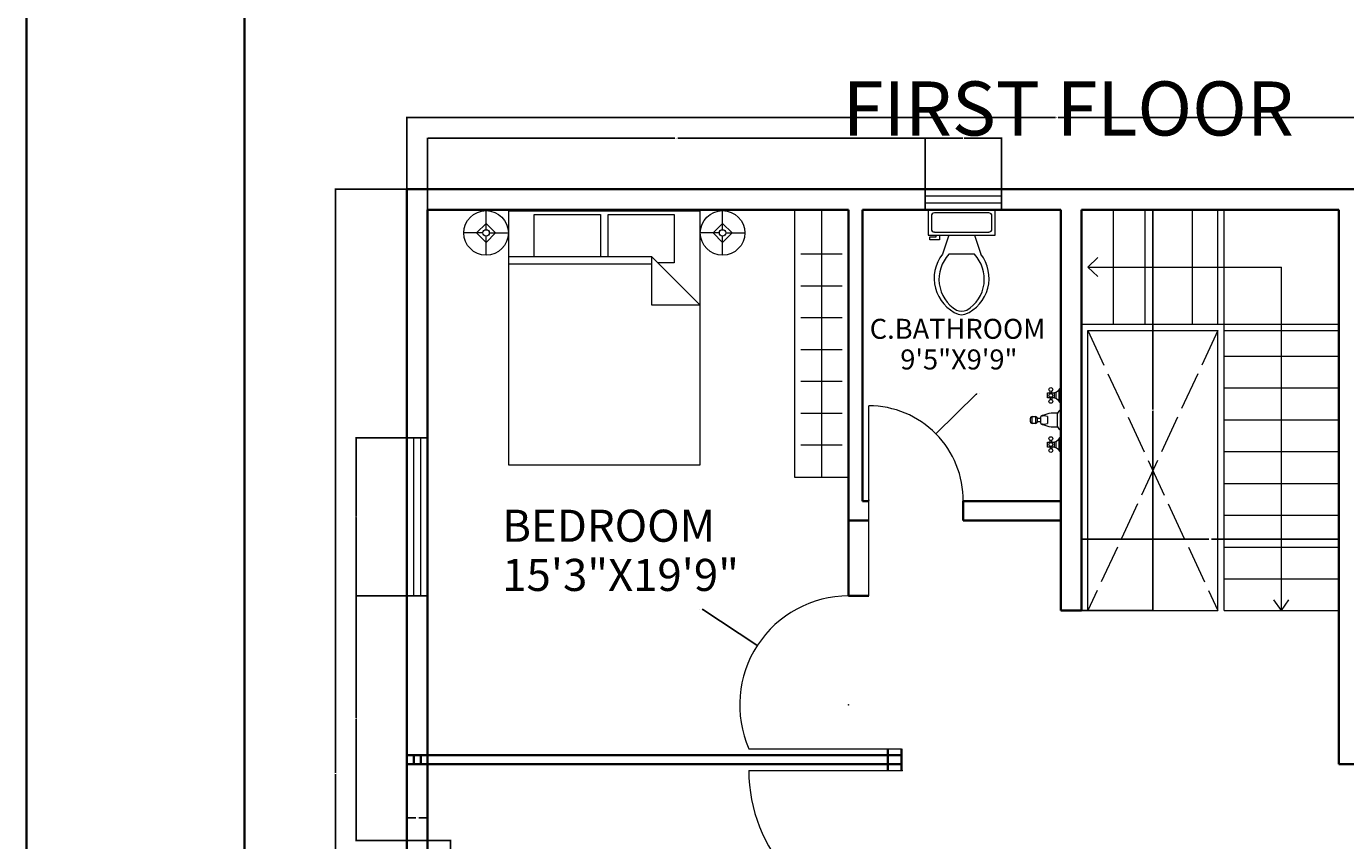
# Model space of a CAD drawing. Units: inches. Extents: x 2286 to 3750, y 1240 to 2345.
# Tile 2 of 7: x 2286 to 2701, y 1537 to 1793. Entities that reach past the tile are written whole.
import ezdxf

# ---------------------------------------------------------------- set-up
doc = ezdxf.new("R2010")
doc.units = ezdxf.units.IN
doc.linetypes.add('ACAD_ISO02W100', pattern=[15, 12, -3])
for name, color, linetype, lineweight in [('A-ANNO-DIMS', 2, 'Continuous', 18), ('A-ANNO-TEXT', 7, 'Continuous', 35), ('A-AREA-IDEN', 7, 'Continuous', 18), ('A-DOOR', 4, 'Continuous', 18), ('A-FLOR-CASE', 8, 'Continuous', 18), ('A-FLOR-FIXT', 9, 'Continuous', 18), ('A-FLOR-STRS', 7, 'Continuous', 18), ('A-FLOR-STRS-HIDN', 8, 'ACAD_ISO02W100', 13), ('A-FURN', 8, 'Continuous', 18), ('A-GLAZ', 51, 'Continuous', 18), ('A-WALL', 7, 'Continuous', 35)]:
    doc.layers.add(name, color=color, linetype=linetype, lineweight=lineweight)
doc.styles.get("Standard").update_dxf_attribs({"font": 'arial.ttf'})
doc.dimstyles.get("Standard").update_dxf_attribs({"dimtxt": 0.18, "dimasz": 0.18, "dimexe": 0.18, "dimexo": 0.0625, "dimgap": 0.09, "dimtad": 0, "dimtih": 1, "dimtoh": 1, "dimdec": 4, "dimzin": 0, "dimdsep": 46, "dimtxsty": 'Standard', "dimcen": 0.09, "dimadec": 0, "dimazin": 0, "dimtfac": 1, "dimtdec": 4, "dimtofl": 0, "dimtmove": 0, "dimatfit": 3, "dimfxl": 1, "dimtolj": 1, "dimtzin": 0, "dimarcsym": 0})

# ---------------------------------------------------------------- blocks, each defined once
blk = doc.blocks.new('Toilet - top')
for p, q in [((9.5, -6), (9.5, -2)), ((-8, -8.5), (-8, -8)), ((-7, -8), (-7, -9.5)), ((-4, -8), (-6, -14)), ((4, -8), (6, -14)), ((-10, -8.5), (-8, -8.5)), ((-10, -9.5), (-10, -8.5)), ((-7, -9.5), (-10, -9.5)), ((4, -14), (-4, -14))]:
    blk.add_line(p, q)
blk.add_lwpolyline([(10.5, -8), (10.5, 0), (-10.5, 0), (-10.5, -8)], close=True)
for points in [[(-9.5, -2), (-9.5, -6)], [(8.5, -1), (-8.5, -1)], [(-8.5, -7), (8.5, -7)]]:
    blk.add_lwpolyline(points)
for centre, radius, start, end in [((-8.62, -1.88), 0.884, 81.8699, 188.1301), ((8.62, -1.88), 0.884, 351.8699, 98.1301), ((-8.62, -6.12), 0.884, 171.8699, 278.1301), ((8.62, -6.12), 0.884, 261.8699, 8.1301), ((3.52, -21.58), 12.17, 141.4691, 247.9714), ((4.2, -21.82), 11.33, 136.3677, 238.9468), ((-3.52, -21.58), 12.17, 292.0284, 38.5307), ((-4.2, -21.82), 11.33, 301.053, 43.6321), ((0, -27.88), 4, 245.7318, 294.2682), ((0, -29), 4, 254.8605, 285.1395)]:
    blk.add_arc(centre, radius, start, end)
blk = doc.blocks.new('Bed - Queen')
for p, q in [((0, -80.00003), (0, 0)), ((0, 0), (59.99999, 0)), ((59.99999, 0), (59.99999, -80.00003)), ((7.99999, -1.2), (28.79998, -1.2)), ((7.99999, -14.4), (7.99999, -1.2)), ((28.79998, -1.2), (28.79998, -14.4)), ((31.19999, -1.2), (51.99999, -1.2)), ((31.19999, -14.4), (31.19999, -1.2)), ((51.99999, -1.2), (51.99999, -16.4)), ((0, -14.4), (44.8, -14.4)), ((59.99999, -29.6), (44.8, -14.4)), ((44.8, -14.4), (44.8, -29.6)), ((51.99999, -16.4), (46.79936, -16.4)), ((44.8, -16.8), (0, -16.8)), ((44.8, -29.6), (59.99999, -29.6)), ((59.99999, -80.00003), (0, -80.00003))]:
    blk.add_line(p, q)
blk = doc.blocks.new('Lamp - Table')
for p, q in [((0, 7), (0, 1)), ((-1, 0), (-7, 0)), ((0, 3), (-3, 0)), ((-3, 0), (0, -3)), ((3, 0), (0, 3)), ((0, -3), (3, 0)), ((1, 0), (7, 0)), ((0, -1), (0, -7))]:
    blk.add_line(p, q)
for radius in [7, 1]:
    blk.add_circle((0, 0), radius)
blk = doc.blocks.new('Faucet - Bathroom front')
for p, q in [((-0.5, 4.25), (0.5, 4.25)), ((0.5, 3.75), (-0.5, 3.75)), ((-0.5, 3), (0.5, 3)), ((0.5, 2), (-0.5, 2)), ((-0.25, 3), (-0.25, 3.5)), ((0.25, 3.5), (0.25, 3)), ((-5, 0), (-2.25, 0)), ((-4.5087, 0.25), (-2.7408, 0.25)), ((-4, 1.625), (-4.25, 1.625)), ((-4, 1.375), (-4.25, 1.375)), ((-3.1442, 0.75), (-4.0979, 0.75)), ((-3.25, 1.625), (-3, 1.625)), ((-3.25, 1.375), (-3, 1.375)), ((-1.5, 0), (1.5, 0)), ((-1, 0.5), (1, 0.5)), ((2.25, 0), (5, 0)), ((2.7413, 0.25), (4.5092, 0.25)), ((3.25, 1.625), (3, 1.625)), ((3.25, 1.375), (3, 1.375)), ((4.1058, 0.75), (3.1521, 0.75)), ((4, 1.625), (4.25, 1.625)), ((4, 1.375), (4.25, 1.375))]:
    blk.add_line(p, q)
for points in [[(-0.5, 3.75), (-0.5, 4.25)], [(-0.25, 4.5), (0.25, 4.5)], [(0.5, 4.25), (0.5, 3.75)], [(0.25, 3.5), (-0.25, 3.5)]]:
    blk.add_lwpolyline(points)
for points in [[(-4, 1), (-4, 2), (-3.25, 2), (-3.25, 1)], [(3.25, 1), (3.25, 2), (4, 2), (4, 1)]]:
    blk.add_lwpolyline(points, close=True)
for centre in [(-4.5, 1.5), (-3.625, 1.5), (-2.75, 1.5), (2.75, 1.5), (3.625, 1.5), (4.5, 1.5)]:
    blk.add_circle(centre, 0.2795)
for centre, radius, start, end in [((-0.2575, 4.2575), 0.2426, 88.22243, 181.7776), ((0.2575, 4.2575), 0.2426, 358.2224, 91.77757), ((3, 1), 4.0311, 150.2551, 187.125), ((0.6413, 2.5), 1.246, 156.3417, 203.6583), ((-0.2575, 3.7425), 0.2426, 178.2224, 271.7776), ((0.2575, 3.7425), 0.2426, 268.2224, 1.777565), ((-3, 1), 4.0311, 352.875, 29.74488), ((-0.6413, 2.5), 1.246, 336.3417, 23.65835), ((-5.375, 1.375), 1.4252, 285.2551, 344.7449), ((-1.875, 1.375), 1.4252, 195.2551, 254.7449), ((-0.7962, -0.2038), 0.7327, 106.1502, 163.8498), ((0.7962, -0.2038), 0.7327, 16.1502, 73.84979), ((1.875, 1.375), 1.4252, 285.2551, 344.7449), ((5.375, 1.375), 1.4252, 195.2551, 254.7449)]:
    blk.add_arc(centre, radius, start, end)
blk = doc.blocks.new('CLOSET-RAIL-84')
for p, q in [((6.5, 0), (6.5, 84)), ((0, 74), (13, 74)), ((0, 64), (13, 64)), ((0, 54), (13, 54)), ((0, 44), (13, 44)), ((0, 34), (13, 34)), ((0, 24), (13, 24)), ((0, 14), (13, 14))]:
    blk.add_line(p, q)
blk = doc.blocks.new('*D36')
at = {"layer": 'A-ANNO-DIMS', "color": 0, "lineweight": -2, "transparency": 16777216}
for p, q in [((2412.36, 1536.75), (2419.68, 1536.75)), ((2419.5, 1536.57), (2419.5, 1512.93)), ((2419.5, 1488.93), (2419.5, 1512.56)), ((2412.36, 1488.75), (2419.68, 1488.75))]:
    blk.add_line(p, q, dxfattribs=at)
at = {"layer": 'A-ANNO-DIMS', "color": 0, "transparency": 16777216}
for points in [[(2419.47, 1536.57), (2419.53, 1536.57), (2419.5, 1536.75)], [(2419.47, 1488.93), (2419.53, 1488.93), (2419.5, 1488.75)]]:
    blk.add_solid(points, dxfattribs=at)
at = {"layer": 'Defpoints', "color": 0, "transparency": 16777216}
for p in [(2412.3, 1536.75), (2419.5, 1536.75), (2412.3, 1488.75)]:
    blk.add_point(p, dxfattribs=at)
at = {"layer": 'A-ANNO-DIMS', "color": 0, "transparency": 16777216, "insert": (2419.5, 1512.75), "char_height": 0.18, "attachment_point": 5}
blk.add_mtext('\\A1;WINDOW 48 TYP.', dxfattribs=at)
blk = doc.blocks.new('*D37')
at = {"layer": 'A-ANNO-DIMS', "color": 0, "lineweight": -2, "transparency": 16777216}
for p, q in [((2405.79, 1536.81), (2405.79, 1544.13)), ((2405.97, 1543.95), (2408.59, 1543.95)), ((2412.12, 1543.95), (2409.5, 1543.95)), ((2412.3, 1536.81), (2412.3, 1544.13))]:
    blk.add_line(p, q, dxfattribs=at)
at = {"layer": 'A-ANNO-DIMS', "color": 0, "transparency": 16777216}
for points in [[(2405.97, 1543.98), (2405.97, 1543.92), (2405.79, 1543.95)], [(2412.12, 1543.98), (2412.12, 1543.92), (2412.3, 1543.95)]]:
    blk.add_solid(points, dxfattribs=at)
at = {"layer": 'Defpoints', "color": 0, "transparency": 16777216}
for p in [(2405.79, 1543.95), (2405.79, 1536.75), (2412.3, 1536.75)]:
    blk.add_point(p, dxfattribs=at)
at = {"layer": 'A-ANNO-DIMS', "color": 0, "transparency": 16777216, "insert": (2409.04, 1543.95), "char_height": 0.18, "attachment_point": 5}
blk.add_mtext('\\A1;7 TYP.', dxfattribs=at)
blk = doc.blocks.new('*D75')
at = {"layer": 'A-ANNO-DIMS', "color": 0, "lineweight": -2, "transparency": 16777216}
for p, q in [((2405.73, 1741.53), (2383.16, 1741.53)), ((2383.34, 1741.35), (2383.34, 1558.04)), ((2383.34, 1374.36), (2383.34, 1557.67)), ((2405.73, 1374.18), (2383.16, 1374.18))]:
    blk.add_line(p, q, dxfattribs=at)
at = {"layer": 'A-ANNO-DIMS', "color": 0, "transparency": 16777216}
for points in [[(2383.31, 1741.35), (2383.37, 1741.35), (2383.34, 1741.53)], [(2383.31, 1374.36), (2383.37, 1374.36), (2383.34, 1374.18)]]:
    blk.add_solid(points, dxfattribs=at)
at = {"layer": 'Defpoints', "color": 0, "transparency": 16777216}
for p in [(2383.34, 1741.53), (2405.79, 1741.53), (2405.79, 1374.18)]:
    blk.add_point(p, dxfattribs=at)
at = {"layer": 'A-ANNO-DIMS', "color": 0, "transparency": 16777216, "insert": (2383.34, 1557.85), "char_height": 0.18, "attachment_point": 5}
blk.add_mtext('\\A1;367.35', dxfattribs=at)
blk = doc.blocks.new('*D76')
at = {"layer": 'A-ANNO-DIMS', "color": 0, "lineweight": -2, "transparency": 16777216}
for p, q in [((2405.79, 1741.59), (2405.79, 1764.22)), ((2405.97, 1764.04), (2609.67, 1764.04)), ((2814.17, 1764.04), (2610.47, 1764.04)), ((2814.35, 1741.59), (2814.35, 1764.22))]:
    blk.add_line(p, q, dxfattribs=at)
at = {"layer": 'A-ANNO-DIMS', "color": 0, "transparency": 16777216}
for points in [[(2405.97, 1764.07), (2405.97, 1764.01), (2405.79, 1764.04)], [(2814.17, 1764.07), (2814.17, 1764.01), (2814.35, 1764.04)]]:
    blk.add_solid(points, dxfattribs=at)
at = {"layer": 'Defpoints', "color": 0, "transparency": 16777216}
for p in [(2814.35, 1764.04), (2405.79, 1741.53), (2814.35, 1741.53)]:
    blk.add_point(p, dxfattribs=at)
at = {"layer": 'A-ANNO-DIMS', "color": 0, "transparency": 16777216, "insert": (2610.07, 1764.04), "char_height": 0.18, "attachment_point": 5}
blk.add_mtext('\\A1;408.6', dxfattribs=at)
blk = doc.blocks.new('*D78')
at = {"layer": 'A-ANNO-DIMS', "color": 0, "lineweight": -2, "transparency": 16777216}
for p, q in [((2617.83, 1609.08), (2617.83, 1631.65)), ((2618.01, 1631.47), (2657.85, 1631.47)), ((2698.47, 1631.47), (2658.64, 1631.47)), ((2698.65, 1609.08), (2698.65, 1631.65))]:
    blk.add_line(p, q, dxfattribs=at)
at = {"layer": 'A-ANNO-DIMS', "color": 0, "transparency": 16777216}
for points in [[(2618.01, 1631.5), (2618.01, 1631.44), (2617.83, 1631.47)], [(2698.47, 1631.5), (2698.47, 1631.44), (2698.65, 1631.47)]]:
    blk.add_solid(points, dxfattribs=at)
at = {"layer": 'Defpoints', "color": 0, "transparency": 16777216}
for p in [(2698.65, 1631.47), (2617.83, 1609.02), (2698.65, 1609.02)]:
    blk.add_point(p, dxfattribs=at)
at = {"layer": 'A-ANNO-DIMS', "color": 0, "transparency": 16777216, "insert": (2658.24, 1631.47), "char_height": 0.18, "attachment_point": 5}
blk.add_mtext('\\A1;80.82', dxfattribs=at)
blk = doc.blocks.new('*D79')
at = {"layer": 'A-ANNO-DIMS', "color": 0, "lineweight": -2, "transparency": 16777216}
for p, q in [((2617.89, 1735.02), (2640.46, 1735.02)), ((2640.28, 1734.84), (2640.28, 1672.2)), ((2640.28, 1609.2), (2640.28, 1671.84)), ((2617.89, 1609.02), (2640.46, 1609.02))]:
    blk.add_line(p, q, dxfattribs=at)
at = {"layer": 'A-ANNO-DIMS', "color": 0, "transparency": 16777216}
for points in [[(2640.25, 1734.84), (2640.31, 1734.84), (2640.28, 1735.02)], [(2640.25, 1609.2), (2640.31, 1609.2), (2640.28, 1609.02)]]:
    blk.add_solid(points, dxfattribs=at)
at = {"layer": 'Defpoints', "color": 0, "transparency": 16777216}
for p in [(2617.83, 1735.02), (2617.83, 1609.02), (2640.28, 1609.02)]:
    blk.add_point(p, dxfattribs=at)
at = {"layer": 'A-ANNO-DIMS', "color": 0, "transparency": 16777216, "insert": (2640.28, 1672.02), "char_height": 0.18, "attachment_point": 5}
blk.add_mtext('\\A1;126', dxfattribs=at)
blk = doc.blocks.new('*D83')
at = {"layer": 'A-ANNO-DIMS', "color": 0, "lineweight": -2, "transparency": 16777216}
for p, q in [((2412.23, 1613.64), (2389.67, 1613.64)), ((2389.85, 1613.46), (2389.85, 1575.37)), ((2389.85, 1536.93), (2389.85, 1575.01)), ((2412.23, 1536.75), (2389.67, 1536.75))]:
    blk.add_line(p, q, dxfattribs=at)
at = {"layer": 'A-ANNO-DIMS', "color": 0, "transparency": 16777216}
for points in [[(2389.82, 1613.46), (2389.88, 1613.46), (2389.85, 1613.64)], [(2389.82, 1536.93), (2389.88, 1536.93), (2389.85, 1536.75)]]:
    blk.add_solid(points, dxfattribs=at)
at = {"layer": 'Defpoints', "color": 0, "transparency": 16777216}
for p in [(2389.85, 1613.64), (2412.3, 1613.64), (2412.3, 1536.75)]:
    blk.add_point(p, dxfattribs=at)
at = {"layer": 'A-ANNO-DIMS', "color": 0, "transparency": 16777216, "insert": (2389.85, 1575.19), "char_height": 0.18, "attachment_point": 5}
blk.add_mtext('\\A1;76.9', dxfattribs=at)
blk = doc.blocks.new('*D84')
at = {"layer": 'A-ANNO-DIMS', "color": 0, "lineweight": -2, "transparency": 16777216}
for p, q in [((2412.23, 1663.29), (2389.67, 1663.29)), ((2389.85, 1663.11), (2389.85, 1638.65)), ((2389.85, 1613.82), (2389.85, 1638.28)), ((2412.23, 1613.64), (2389.67, 1613.64))]:
    blk.add_line(p, q, dxfattribs=at)
at = {"layer": 'A-ANNO-DIMS', "color": 0, "transparency": 16777216}
for points in [[(2389.82, 1663.11), (2389.88, 1663.11), (2389.85, 1663.29)], [(2389.82, 1613.82), (2389.88, 1613.82), (2389.85, 1613.64)]]:
    blk.add_solid(points, dxfattribs=at)
at = {"layer": 'Defpoints', "color": 0, "transparency": 16777216}
for p in [(2389.85, 1663.29), (2412.3, 1663.29), (2412.3, 1613.64)]:
    blk.add_point(p, dxfattribs=at)
at = {"layer": 'A-ANNO-DIMS', "color": 0, "transparency": 16777216, "insert": (2389.85, 1638.47), "char_height": 0.18, "attachment_point": 5}
blk.add_mtext('\\A1;49.65', dxfattribs=at)
blk = doc.blocks.new('*D85')
at = {"layer": 'A-ANNO-DIMS', "color": 0, "lineweight": -2, "transparency": 16777216}
for p, q in [((2412.3, 1735.08), (2412.29, 1757.65)), ((2412.47, 1757.47), (2490.04, 1757.5)), ((2568.53, 1757.53), (2490.95, 1757.5)), ((2568.72, 1735.15), (2568.71, 1757.71))]:
    blk.add_line(p, q, dxfattribs=at)
at = {"layer": 'A-ANNO-DIMS', "color": 0, "transparency": 16777216}
for points in [[(2412.47, 1757.5), (2412.47, 1757.44), (2412.29, 1757.47)], [(2568.53, 1757.56), (2568.53, 1757.5), (2568.71, 1757.53)]]:
    blk.add_solid(points, dxfattribs=at)
at = {"layer": 'Defpoints', "color": 0, "transparency": 16777216}
for p in [(2568.71, 1757.53), (2412.3, 1735.02), (2568.72, 1735.08)]:
    blk.add_point(p, dxfattribs=at)
at = {"layer": 'A-ANNO-DIMS', "color": 0, "transparency": 16777216, "insert": (2490.5, 1757.5), "char_height": 0.18, "attachment_point": 5}
blk.add_mtext('\\A1;156.42', dxfattribs=at)
blk = doc.blocks.new('*D86')
at = {"layer": 'A-ANNO-DIMS', "color": 0, "lineweight": -2, "transparency": 16777216}
for p, q in [((2568.72, 1735.15), (2568.72, 1757.71)), ((2568.9, 1757.53), (2580.5, 1757.53)), ((2592.54, 1757.53), (2580.94, 1757.53)), ((2592.72, 1735.15), (2592.72, 1757.71))]:
    blk.add_line(p, q, dxfattribs=at)
at = {"layer": 'A-ANNO-DIMS', "color": 0, "transparency": 16777216}
for points in [[(2568.9, 1757.56), (2568.9, 1757.5), (2568.72, 1757.53)], [(2592.54, 1757.56), (2592.54, 1757.5), (2592.72, 1757.53)]]:
    blk.add_solid(points, dxfattribs=at)
at = {"layer": 'Defpoints', "color": 0, "transparency": 16777216}
for p in [(2592.72, 1757.53), (2568.72, 1735.08), (2592.72, 1735.08)]:
    blk.add_point(p, dxfattribs=at)
at = {"layer": 'A-ANNO-DIMS', "color": 0, "transparency": 16777216, "insert": (2580.72, 1757.53), "char_height": 0.18, "attachment_point": 5}
blk.add_mtext('\\A1;24', dxfattribs=at)
blk = doc.blocks.new('*D128')
at = {"layer": 'A-ANNO-DIMS', "color": 0, "lineweight": -2, "transparency": 16777216}
for p, q in [((2561.39, 1558.75), (2561.57, 1558.75)), ((2561.48, 1558.66), (2561.48, 1558.84)), ((2504.41, 1506.84), (2525.67, 1526.18)), ((2504.23, 1506.84), (2504.41, 1506.84))]:
    blk.add_line(p, q, dxfattribs=at)
at = {"layer": 'A-ANNO-DIMS', "color": 0, "transparency": 16777216}
blk.add_solid([(2525.65, 1526.2), (2525.69, 1526.16), (2525.81, 1526.3)], dxfattribs=at)
at = {"layer": 'Defpoints', "color": 0, "transparency": 16777216}
for p in [(2561.48, 1558.75), (2525.81, 1526.3)]:
    blk.add_point(p, dxfattribs=at)
at = {"layer": 'A-ANNO-DIMS', "color": 0, "transparency": 16777216, "insert": (2503.75, 1506.84), "char_height": 0.18, "attachment_point": 5}
blk.add_mtext('\\A1;R48.22', dxfattribs=at)
blk = doc.blocks.new('*D130')
at = {"layer": 'A-ANNO-DIMS', "color": 0, "lineweight": -2, "transparency": 16777216}
for p, q in [((2498.58, 1609.37), (2498.76, 1609.37)), ((2498.76, 1609.37), (2515.81, 1598.22)), ((2544.54, 1579.39), (2544.72, 1579.39)), ((2544.63, 1579.3), (2544.63, 1579.48))]:
    blk.add_line(p, q, dxfattribs=at)
at = {"layer": 'A-ANNO-DIMS', "color": 0, "transparency": 16777216}
blk.add_solid([(2515.82, 1598.25), (2515.79, 1598.2), (2515.96, 1598.13)], dxfattribs=at)
at = {"layer": 'Defpoints', "color": 0, "transparency": 16777216}
for p in [(2515.96, 1598.13), (2544.63, 1579.39)]:
    blk.add_point(p, dxfattribs=at)
at = {"layer": 'A-ANNO-DIMS', "color": 0, "transparency": 16777216, "insert": (2498.1, 1609.37), "char_height": 0.18, "attachment_point": 5}
blk.add_mtext('\\A1;R34.25', dxfattribs=at)
blk = doc.blocks.new('*D132')
at = {"layer": 'A-ANNO-DIMS', "color": 0, "lineweight": -2, "transparency": 16777216}
for p, q in [((2584.72, 1677.1), (2572.19, 1664.72)), ((2584.9, 1677.1), (2584.72, 1677.1)), ((2550.88, 1643.73), (2551.06, 1643.73)), ((2550.97, 1643.64), (2550.97, 1643.82))]:
    blk.add_line(p, q, dxfattribs=at)
at = {"layer": 'A-ANNO-DIMS', "color": 0, "transparency": 16777216}
blk.add_solid([(2572.17, 1664.74), (2572.21, 1664.69), (2572.06, 1664.59)], dxfattribs=at)
at = {"layer": 'Defpoints', "color": 0, "transparency": 16777216}
for p in [(2572.06, 1664.59), (2550.97, 1643.73)]:
    blk.add_point(p, dxfattribs=at)
at = {"layer": 'A-ANNO-DIMS', "color": 0, "transparency": 16777216, "insert": (2585.45, 1677.1), "char_height": 0.18, "attachment_point": 5}
blk.add_mtext('\\A1;R29.663', dxfattribs=at)

msp = doc.modelspace()

# ---------------------------------------------------------------- linework, layer by layer
at = {"layer": 'A-DOOR'}
for p, q in [((2550.967, 1613.6385), (2550.967, 1673.397)), ((2513.2601, 1565.6385), (2561.2601, 1565.6385)), ((2513.2601, 1558.746), (2561.2601, 1558.746))]:
    msp.add_line(p, q, dxfattribs=at)
for centre, radius, start, end in [((2550.967, 1643.7338), 29.6632, 359.349399, 90), ((2544.6283, 1579.3889), 34.2496, 90, 203.67046), ((2561.4757, 1558.746), 48.2156, 180, 264.579918)]:
    msp.add_arc(centre, radius, start, end, dxfattribs=at)
at = {"layer": 'A-FLOR-CASE'}
for p, q in [((2544.6283, 1735.0185), (2527.6283, 1735.0185)), ((2527.6283, 1735.0185), (2527.6283, 1651.0185)), ((2544.6283, 1735.0185), (2544.6283, 1651.0185)), ((2527.6283, 1651.0185), (2544.6283, 1651.0185))]:
    msp.add_line(p, q, dxfattribs=at)
at = {"layer": 'A-FLOR-STRS'}
for p, q in [((2627.8314, 1699.0185), (2627.8314, 1735.0185)), ((2637.8314, 1699.0185), (2637.8314, 1735.0185)), ((2652.6534, 1699.0185), (2652.6534, 1735.0185)), ((2660.6534, 1699.0185), (2660.6534, 1735.0185)), ((2662.6534, 1609.0185), (2662.6534, 1735.0185)), ((2619.8314, 1717.0185), (2622.9458, 1720.0095)), ((2619.8314, 1717.0185), (2680.6534, 1717.0185)), ((2619.8314, 1717.0185), (2622.9458, 1714.0275)), ((2680.6534, 1609.0185), (2680.6534, 1717.0185)), ((2617.8314, 1699.0185), (2698.6534, 1699.0185)), ((2619.8314, 1697.0185), (2660.6534, 1697.0185)), ((2619.8314, 1609.0185), (2619.8314, 1697.0185)), ((2660.6534, 1609.0185), (2660.6534, 1697.0185)), ((2662.6534, 1697.0185), (2698.6534, 1697.0185)), ((2662.6534, 1689.0185), (2698.6534, 1689.0185)), ((2662.6534, 1679.0185), (2698.6534, 1679.0185)), ((2662.6534, 1669.0185), (2698.6534, 1669.0185)), ((2662.6534, 1659.0185), (2698.6534, 1659.0185)), ((2662.6534, 1649.0185), (2698.6534, 1649.0185)), ((2662.6534, 1639.0185), (2698.6534, 1639.0185)), ((2662.6534, 1629.0185), (2698.6534, 1629.0185)), ((2662.6534, 1619.0185), (2698.6534, 1619.0185)), ((2619.8314, 1609.0185), (2660.6534, 1609.0185)), ((2662.6534, 1609.0185), (2698.6534, 1609.0185)), ((2680.6534, 1609.0185), (2678.2985, 1612.434)), ((2680.6534, 1609.0185), (2683.0082, 1612.434))]:
    msp.add_line(p, q, dxfattribs=at)
at = {"layer": 'A-FLOR-STRS-HIDN'}
for p, q in [((2619.8314, 1697.0185), (2660.6534, 1609.0185)), ((2660.6534, 1697.0185), (2619.8314, 1609.0185))]:
    msp.add_line(p, q, dxfattribs=at)
at = {"layer": 'A-GLAZ'}
for p, q in [((2568.7168, 1735.0833), (2568.7168, 1741.5914)), ((2592.7168, 1735.0833), (2592.7168, 1741.5914)), ((2568.7168, 1739.3666), (2592.7168, 1739.3666)), ((2568.7168, 1737.1785), (2592.7168, 1737.1785)), ((2405.7888, 1663.2921), (2412.2969, 1663.2921)), ((2407.9488, 1613.6385), (2407.9488, 1663.2921)), ((2410.1369, 1613.6385), (2410.1369, 1663.2921)), ((2405.7888, 1613.6385), (2412.2969, 1613.6385))]:
    msp.add_line(p, q, dxfattribs=at)
at = {"layer": 'A-WALL'}
for p, q in [((2405.7888, 1741.5266), (2814.3529, 1741.5266)), ((2405.7888, 1374.1804), (2405.7888, 1741.5266)), ((2412.2969, 1735.0185), (2544.6283, 1735.0185)), ((2412.2969, 1380.6885), (2412.2969, 1735.0185)), ((2412.2969, 1674.2762), (2412.2969, 1735.0185)), ((2544.6283, 1613.6385), (2544.6283, 1735.0185)), ((2548.967, 1643.397), (2548.967, 1735.0185)), ((2548.967, 1735.0185), (2611.3233, 1735.0185)), ((2611.3233, 1609.0185), (2611.3233, 1735.0185)), ((2617.8314, 1609.0185), (2617.8314, 1735.0185)), ((2617.8314, 1735.0185), (2698.6534, 1735.0185)), ((2698.6534, 1560.746), (2698.6534, 1735.0185)), ((2548.967, 1643.397), (2550.967, 1643.397)), ((2580.6283, 1637.397), (2580.6283, 1643.397)), ((2580.6283, 1643.397), (2611.3233, 1643.397)), ((2544.6283, 1637.397), (2550.967, 1637.397)), ((2580.6283, 1637.397), (2611.3233, 1637.397)), ((2544.6283, 1613.6385), (2550.967, 1613.6385)), ((2611.3233, 1609.0185), (2617.8314, 1609.0185)), ((2405.7888, 1563.6385), (2561.2601, 1563.6385)), ((2407.9488, 1560.746), (2407.9488, 1563.6385)), ((2410.1369, 1560.746), (2410.1369, 1563.6385)), ((2556.9214, 1558.746), (2556.9214, 1565.6385)), ((2561.2601, 1558.746), (2561.2601, 1565.6385)), ((2405.7888, 1560.746), (2561.2601, 1560.746)), ((2698.6534, 1560.746), (2704.9921, 1560.746))]:
    msp.add_line(p, q, dxfattribs=at)
for points in [[(2286.2079, 2344.8717), (3750.2574, 2344.8717), (3750.2574, 1240.4105), (2286.2079, 1240.4105)], [(2354.794, 2286.8809), (3673.7575, 2286.8809), (3673.7575, 1335.3046), (2354.794, 1335.3046)]]:
    msp.add_lwpolyline(points, close=True, dxfattribs=at)

# ---------------------------------------------------------------- block references
at = {"layer": 'A-FLOR-CASE', "rotation": 180}
msp.add_blockref('CLOSET-RAIL-84', (2542.6283, 1735.0185), dxfattribs=at)
at = {"layer": 'A-FLOR-FIXT'}
msp.add_blockref('Toilet - top', (2580.1452, 1735.0185), dxfattribs=at)
at = {"layer": 'A-FLOR-FIXT', "xscale": 2.130333955726564, "yscale": 2.130333955726564, "zscale": 2.130333955726564, "rotation": 89.99999999999999}
msp.add_blockref('Faucet - Bathroom front', (2611.3776, 1668.9397), dxfattribs=at)
at = {"layer": 'A-FURN', "rotation": 180}
for p in [(2430.6895, 1727.742), (2505.0052, 1727.742)]:
    msp.add_blockref('Lamp - Table', p, dxfattribs=at)
at = {"layer": 'A-FURN'}
msp.add_blockref('Bed - Queen', (2437.8408, 1734.7097), dxfattribs=at)

# ---------------------------------------------------------------- texts
at = {"layer": 'A-ANNO-TEXT'}
msp.add_text('FIRST FLOOR', height=17, dxfattribs=at).set_placement((2542.7553, 1758.3416))
at = {"layer": 'A-AREA-IDEN'}
for s, height, p in [(' C.BATHROOM', 6.282441, (2549.3366, 1694.4492)), ('      9\'5"X9\'9"', 6.282441, (2549.3366, 1684.8207)), ('BEDROOM', 10.08366, (2435.7677, 1630.6606)), ('15\'3"X19\'9"', 10.083661, (2435.7677, 1615.2064))]:
    msp.add_text(s, height=height, dxfattribs=at).set_placement(p)

# ---------------------------------------------------------------- dimensions: what is measured, and where the dimension line sits
at = {"layer": 'A-ANNO-DIMS'}
for base, p1, p2, override, picture, middle in [((2814.3529, 1764.0414), (2405.7888, 1741.5266), (2814.3529, 1741.5266), {"dimdec": 1, "dimlfac": 1, "dimrnd": 0, "dimzin": 0, "dimdsep": 46, "dimlunit": 2}, '*D76', (2610.0709, 1764.0414)), ((2592.7168, 1757.5333), (2568.7168, 1735.0833), (2592.7168, 1735.0833), {"dimdec": 0, "dimlfac": 1, "dimrnd": 0, "dimzin": 0, "dimdsep": 46, "dimlunit": 2}, '*D86', (2580.7168, 1757.5333)), ((2698.6534, 1631.4685), (2617.8314, 1609.0185), (2698.6534, 1609.0185), {"dimdec": 2, "dimlfac": 1, "dimrnd": 0, "dimzin": 0, "dimdsep": 46, "dimlunit": 2}, '*D78', (2658.2424, 1631.4685))]:
    dim = msp.add_linear_dim(base=base, p1=p1, p2=p2, dimstyle='Standard', override=override, dxfattribs=at)
    dim.commit()
    dim.dimension.update_dxf_attribs({"geometry": picture, "text_midpoint": middle})
for base, p1, p2, angle, override, picture, middle in [((2568.7075, 1757.5333), (2412.2969, 1735.0185), (2568.7168, 1735.0833), 0.023747, {"dimdec": 2, "dimlfac": 1, "dimrnd": 0, "dimzin": 0, "dimdsep": 46, "dimlunit": 2}, '*D85', (2490.4976, 1757.5009)), ((2383.3388, 1741.5266), (2405.7888, 1374.1804), (2405.7888, 1741.5266), 90, {"dimdec": 2, "dimlfac": 1, "dimrnd": 0, "dimzin": 0, "dimdsep": 46, "dimlunit": 2}, '*D75', (2383.3388, 1557.8535)), ((2640.2814, 1609.0185), (2617.8314, 1735.0185), (2617.8314, 1609.0185), 270, {"dimdec": 0, "dimlfac": 1, "dimrnd": 0, "dimzin": 0, "dimdsep": 46, "dimlunit": 2}, '*D79', (2640.2814, 1672.0185)), ((2389.8469, 1663.2921), (2412.2969, 1613.6385), (2412.2969, 1663.2921), 90, {"dimdec": 2, "dimlfac": 1, "dimrnd": 0, "dimzin": 0, "dimdsep": 46, "dimlunit": 2}, '*D84', (2389.8469, 1638.4653)), ((2389.8469, 1613.6385), (2412.2969, 1536.746), (2412.2969, 1613.6385), 90, {"dimdec": 1, "dimlfac": 1, "dimrnd": 0, "dimzin": 0, "dimdsep": 46, "dimlunit": 2}, '*D83', (2389.8469, 1575.1922))]:
    dim = msp.add_linear_dim(base=base, p1=p1, p2=p2, angle=angle, dimstyle='Standard', override=override, dxfattribs=at)
    dim.commit()
    dim.dimension.update_dxf_attribs({"geometry": picture, "text_midpoint": middle})
for center, mpoint, override, picture, middle in [((2550.967, 1643.7338), (2572.0611, 1664.5891), {"dimdec": 3, "dimlfac": 1, "dimrnd": 0, "dimzin": 0, "dimdsep": 46, "dimlunit": 2}, '*D132', (2585.4473, 1677.1023)), ((2544.6283, 1579.3889), (2515.9579, 1598.1251), {"dimdec": 2, "dimlfac": 1, "dimrnd": 0, "dimzin": 0, "dimdsep": 46, "dimlunit": 2}, '*D130', (2498.0952, 1609.3668)), ((2561.4757, 1558.746), (2525.8079, 1526.3029), {"dimdec": 2, "dimlfac": 1, "dimrnd": 0, "dimzin": 0, "dimdsep": 46, "dimlunit": 2}, '*D128', (2503.7483, 1506.8371))]:
    dim = msp.add_radius_dim(center=center, mpoint=mpoint, dimstyle='Standard', override=override, dxfattribs=at)
    dim.commit()
    dim.dimension.update_dxf_attribs({"geometry": picture, "text_midpoint": middle, "dimtype": 164})
for base, p1, p2, angle, text, picture, middle in [((2405.7888, 1543.946), (2412.2969, 1536.746), (2405.7888, 1536.746), 180, '<> TYP.', '*D37', (2409.0428, 1543.946)), ((2419.4969, 1536.746), (2412.2969, 1488.746), (2412.2969, 1536.746), 90, 'WINDOW <> TYP.', '*D36', (2419.4969, 1512.746))]:
    dim = msp.add_linear_dim(base=base, p1=p1, p2=p2, angle=angle, text=text, dimstyle='Standard', override={"dimdec": 0, "dimlfac": 1, "dimrnd": 0, "dimzin": 0, "dimdsep": 46, "dimlunit": 2}, dxfattribs=at)
    dim.commit()
    dim.dimension.update_dxf_attribs({"geometry": picture, "text_midpoint": middle})

doc.saveas('drawing.dxf')
